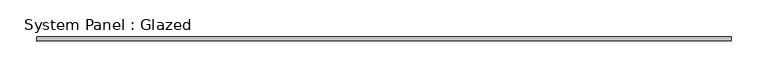
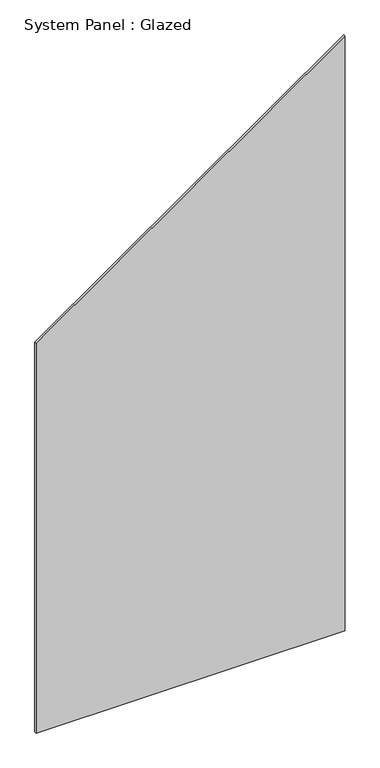
"""IFC4 building model written with IfcOpenShell, lengths in millimetres: plate geometry, System Panel : Glazed."""

from ifc_helpers import new_model, si_unit, frame, origin, place, context, project, spatial, polyline, outline, extrude, source, transform, mapped, element, save


def system_panel_glazed_9142b3e3(model_context):
    return source(origin(), model_context, "Body", "SweptSolid", [
        extrude(outline(polyline([(0.0, -475.0), (0.0, 475.0), (1931.0404197, 475.0), (1265.8432584, -475.0), (0.0, -475.0)])), frame((0.0, 34.0, 0.0), z_axis=(0.0, 1.0, 0.0), x_axis=(0.0, 0.0, 1.0)), (0.0, 0.0, 1.0), 6.0),
    ])


if __name__ == "__main__":
    model = new_model("IFC4")
    model_context = context("Model", 3, world=origin())
    ifc_project = project(units=[si_unit("LENGTHUNIT", "METRE", prefix="MILLI")], contexts=[model_context])
    site = spatial("IfcSite", under=ifc_project)
    building = spatial("IfcBuilding", under=site)
    placement = place(None, origin())
    system_panel_glazed_shape = system_panel_glazed_9142b3e3(model_context)
    element("IfcPlate", 1, ObjectType="System Panel : Glazed", at=placement, inside=building, context=model_context, shape_type="MappedRepresentation", body=[
        mapped(system_panel_glazed_shape, transform((0.0, 0.0, 0.0), x_axis=(1.0, 0.0, 0.0), y_axis=(0.0, 1.0, 0.0), z_axis=(0.0, 0.0, 1.0))),
    ])
    save(model, "model.ifc")

# Revit data of these elements
# Type "System Panel : Glazed"
#   Construction Type Id = "GSP4R"
#   Analytic Construction = "1/8 in Pilkington single glazing"
#   Visual Light Transmittance = 0.9
#   Solar Heat Gain Coefficient = 0.86
#   Heat Transfer Coefficient (U) = 6.7069 W/(m²·K)
#   Define Thermal Properties by = 1
# Element 1 (IfcPlate, "System Panel : Glazed")
#   Materials on its faces: "Default New Material(6)"
# Materials
#   "Default New Material(6)": class "Generic", colour RGB 191 25 25, transparency 0.9, Cost = 0
